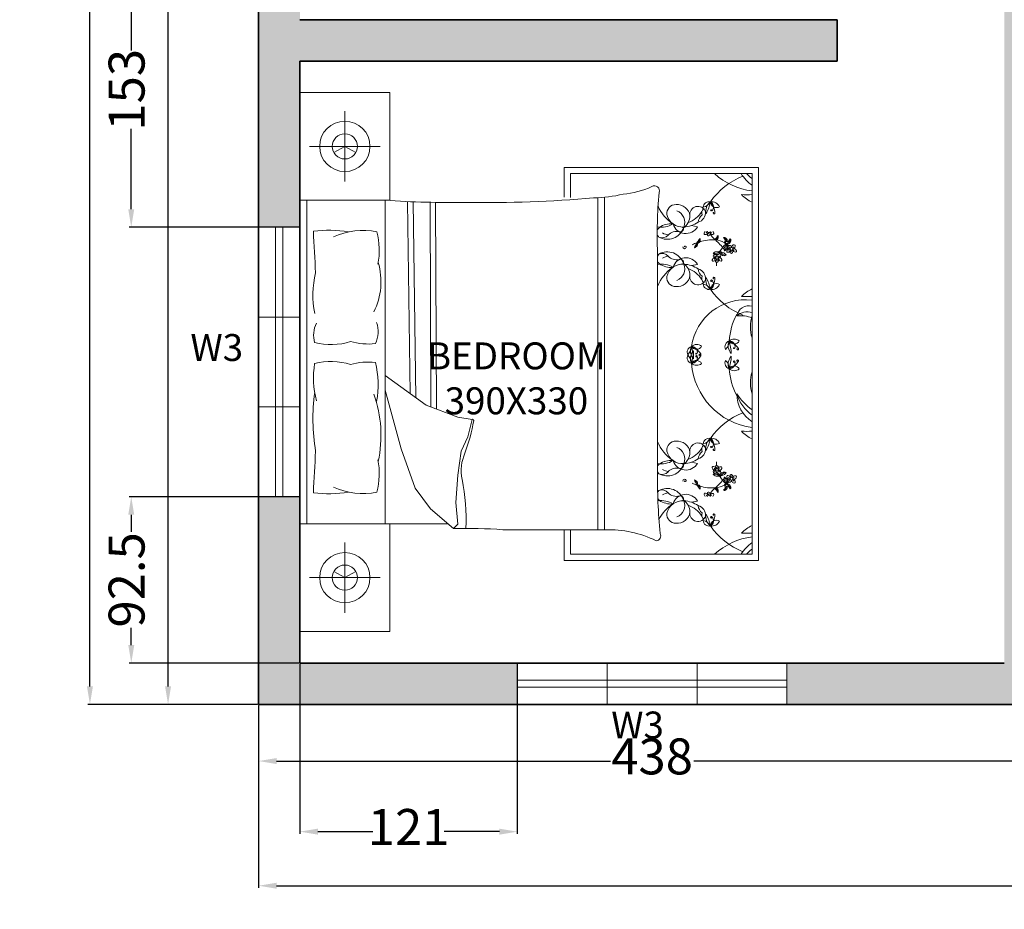
# Model space of a CAD drawing. Units: centimetres. Extents: x 2137 to 3697, y 183 to 2094.
# Tile 1 of 8: x 2137 to 2685, y 183 to 678. Entities that reach past the tile are written whole.
import ezdxf

# ---------------------------------------------------------------- set-up
doc = ezdxf.new("R2010")
doc.units = ezdxf.units.CM
for name, color, linetype, lineweight in [('A-ANNO-DIMS', 2, 'Continuous', 18), ('A-ANNO-TEXT', 7, 'Continuous', 18), ('A-AREA-IDEN', 7, 'Continuous', 25), ('A-FURN', 8, 'Continuous', 18), ('A-GLAZ', 4, 'Continuous', 18), ('A-WALL', 7, 'Continuous', 35), ('A-WALL-PATT', 52, 'Continuous', 13)]:
    doc.layers.add(name, color=color, linetype=linetype, lineweight=lineweight)
doc.styles.get("Standard").update_dxf_attribs({"font": 'arial.ttf'})
doc.dimstyles.new('ISO-25', dxfattribs={"dimtxt": 20, "dimasz": 10, "dimexe": 1.25, "dimexo": 0.625, "dimtad": 0, "dimtxsty": 'Standard', "dimcen": 2.5, "dimadec": 0, "dimazin": 0, "dimtfac": 1, "dimtmove": 0, "dimatfit": 3, "dimfxl": 1, "dimarcsym": 0})

# ---------------------------------------------------------------- blocks, each defined once
blk = doc.blocks.new('*D2')
at = {"layer": 'A-ANNO-DIMS', "color": 0, "lineweight": -2, "transparency": 16777216}
for p, q in [((2270.02, 295.95), (2270.02, 263.76)), ((2708.02, 295.95), (2708.02, 263.76)), ((2280.02, 265.01), (2465.88, 265.01)), ((2698.02, 265.01), (2512.16, 265.01))]:
    blk.add_line(p, q, dxfattribs=at)
at = {"layer": 'A-ANNO-DIMS', "color": 0, "transparency": 16777216}
for points in [[(2280.02, 266.68), (2280.02, 263.35), (2270.02, 265.01)], [(2698.02, 266.68), (2698.02, 263.35), (2708.02, 265.01)]]:
    blk.add_solid(points, dxfattribs=at)
at = {"layer": 'Defpoints', "color": 0, "transparency": 16777216}
for p in [(2270.02, 296.58), (2708.02, 296.58), (2708.02, 265.01)]:
    blk.add_point(p, dxfattribs=at)
at = {"layer": 'A-ANNO-DIMS', "color": 0, "transparency": 16777216, "insert": (2489.02, 265.01), "char_height": 20, "attachment_point": 5}
blk.add_mtext('438', dxfattribs=at)
blk = doc.blocks.new('*D5')
at = {"layer": 'A-ANNO-DIMS', "color": 0, "lineweight": -2, "transparency": 16777216}
for p, q in [((3590.02, 419.95), (3590.02, 194.39)), ((2270.02, 295.95), (2270.02, 194.39)), ((2280.02, 195.64), (2900.51, 195.64)), ((3580.02, 195.64), (2959.54, 195.64))]:
    blk.add_line(p, q, dxfattribs=at)
at = {"layer": 'A-ANNO-DIMS', "color": 0, "transparency": 16777216}
for points in [[(2280.02, 197.31), (2280.02, 193.97), (2270.02, 195.64)], [(3580.02, 197.31), (3580.02, 193.97), (3590.02, 195.64)]]:
    blk.add_solid(points, dxfattribs=at)
at = {"layer": 'Defpoints', "color": 0, "transparency": 16777216}
for p in [(3590.02, 420.58), (2270.02, 296.58), (3590.02, 195.64)]:
    blk.add_point(p, dxfattribs=at)
at = {"layer": 'A-ANNO-DIMS', "color": 0, "transparency": 16777216, "insert": (2930.02, 195.64), "char_height": 20, "attachment_point": 5}
blk.add_mtext('1320', dxfattribs=at)
blk = doc.blocks.new('*D7')
at = {"layer": 'A-ANNO-DIMS', "color": 0, "lineweight": -2, "transparency": 16777216}
for p, q in [((2269.4, 1526.58), (2218.41, 1526.58)), ((2219.66, 1516.58), (2219.66, 941.09)), ((2219.66, 306.58), (2219.66, 882.07)), ((2269.4, 296.58), (2218.41, 296.58))]:
    blk.add_line(p, q, dxfattribs=at)
at = {"layer": 'A-ANNO-DIMS', "color": 0, "transparency": 16777216}
for points in [[(2217.99, 1516.58), (2221.33, 1516.58), (2219.66, 1526.58)], [(2217.99, 306.58), (2221.33, 306.58), (2219.66, 296.58)]]:
    blk.add_solid(points, dxfattribs=at)
at = {"layer": 'Defpoints', "color": 0, "transparency": 16777216}
for p in [(2270.02, 1526.58), (2219.66, 296.58), (2270.02, 296.58)]:
    blk.add_point(p, dxfattribs=at)
at = {"layer": 'A-ANNO-DIMS', "color": 0, "transparency": 16777216, "insert": (2219.66, 911.58), "char_height": 20, "attachment_point": 5, "rotation": 90}
blk.add_mtext('1230', dxfattribs=at)
blk = doc.blocks.new('BED')
for p, q in [((2442.52, 2474.71), (2742.52, 2474.71)), ((2502.52, 2474.71), (2502.52, 2392.37)), ((2472.52, 2430.11), (2472.52, 2469.31)), ((2682.52, 2470.86), (2502.52, 2470.86)), ((2712.52, 2430.11), (2712.52, 2469.31)), ((2492.12, 2449.71), (2452.92, 2449.71)), ((2692.92, 2449.71), (2732.12, 2449.71)), ((2502.52, 2427.3), (2682.52, 2427.3)), ((2544.19, 2418.38), (2576.9, 2427.3)), ((2584.93, 2427.3), (2568.49, 2404.42)), ((2522.31, 2410.49), (2544.19, 2418.38)), ((2681.6, 2411.76), (2572.66, 2410.22)), ((2681.71, 2414.84), (2574.9, 2413.34)), ((2510.77, 2401.99), (2522.31, 2410.49)), ((2499.83, 2389.24), (2510.77, 2401.99)), ((2568.49, 2404.42), (2561.81, 2386.81)), ((2681.44, 2402.31), (2567.52, 2401.86)), ((2681.46, 2399.23), (2566.35, 2398.76)), ((2502.26, 2386.81), (2499.83, 2389.24)), ((2514.41, 2388.02), (2502.26, 2386.81)), ((2529.61, 2386.81), (2514.41, 2388.02)), ((2542.97, 2384.99), (2529.61, 2386.81)), ((2550.87, 2381.34), (2542.97, 2384.99)), ((2561.81, 2386.81), (2560.59, 2378.91)), ((2560.59, 2378.91), (2550.87, 2381.34)), ((2482.11, 2327.65), (2499.08, 2327.65)), ((2482.11, 2219.58), (2482.11, 2327.65)), ((2499.08, 2324.17), (2485.59, 2324.17)), ((2485.59, 2324.17), (2485.59, 2223.06)), ((2697.35, 2324.17), (2684.13, 2324.17)), ((2684.19, 2327.65), (2700.83, 2327.65)), ((2697.35, 2223.06), (2697.35, 2324.17)), ((2700.83, 2327.65), (2700.83, 2219.58)), ((2683.88, 2308.94), (2499.06, 2308.94)), ((2684.17, 2305.2), (2499.06, 2305.2)), ((2653.42, 2275.73), (2531.62, 2275.73)), ((2515.15, 2253.47), (2514.49, 2256.86)), ((2536.12, 2253.47), (2536.78, 2256.86)), ((2646.82, 2253.47), (2646.16, 2256.86)), ((2667.79, 2253.47), (2668.45, 2256.86)), ((2700.83, 2219.58), (2482.11, 2219.58)), ((2485.59, 2223.06), (2697.35, 2223.06))]:
    blk.add_line(p, q)
for points in [[(2502.52, 2424.71), (2442.52, 2424.71), (2442.52, 2474.71)], [(2682.52, 2474.71), (2682.52, 2424.71), (2742.52, 2424.71), (2742.52, 2474.71)], [(2472.52, 2449.71), (2476.02, 2455.77)], [(2712.52, 2449.71), (2709.02, 2455.77)], [(2472.52, 2449.71), (2476.02, 2443.65)], [(2712.52, 2449.71), (2709.02, 2443.65)]]:
    blk.add_lwpolyline(points)
for points in [[(2519.75, 2467.23, 0.074897), (2520.11, 2447.64, -0.472817)], [(2591.11, 2446.54, 0.14099), (2591.71, 2466.53, 0.235245)], [(2603.92, 2446.54, -0.14099), (2603.32, 2466.53, -0.235245)], [(2665.29, 2467.23, -0.074897), (2664.92, 2447.64, 0.472817)], [(2499.2, 2361.77, 0.001242), (2499.06, 2304.85, -0.127202), (2493.05, 2276.48)], [(2683.8, 2311.3, 0.056112), (2685.97, 2294.79, 0.095341), (2690.19, 2278.9)]]:
    blk.add_lwpolyline(points, format="xyb")
for centre, radius in [((2472.52, 2449.71), 14), ((2712.52, 2449.71), 14), ((2472.52, 2449.71), 7), ((2712.52, 2449.71), 7), ((2532.49, 2242.6), 0.764), ((2650.46, 2242.6), 0.764), ((2527.49, 2234.55), 0.764), ((2655.45, 2234.55), 0.764)]:
    blk.add_circle(centre, radius)
for centre, radius, start, end in [((2685.11, 5322.24), 2859.79, 266.68521, 267.14978), ((2560.85, 2358.67), 108.8, 82.2196, 99.497), ((2583.83, 2413.66), 53.46, 81.5249, 103.96), ((2607.44, 2452.27), 14.84, 63.3437, 106.1026), ((2629.68, 2414.74), 52.74, 76.3427, 101.1841), ((2499.93, 5322.24), 2859.79, 272.85022, 273.31479), ((2557.97, 2439.77), 38.67, 155.1316, 191.7583), ((2627.07, 2439.77), 38.67, 348.2417, 24.8684), ((2555.75, 2436.51), 36.76, 354.0129, 15.8293), ((2639.29, 2436.51), 36.76, 164.1707, 185.9871), ((2551.61, 2499.32), 69.73, 258.0397, 289.2615), ((2637.23, 2467.78), 38.19, 243.8761, 286.1746), ((2530.45, 2470.74), 40.2, 255.1039, 281.0369), ((2579.84, 2484.1), 52.9, 259.8617, 283.6238), ((2609.45, 2447.1), 15.9, 245.0183, 288.5407), ((2654.58, 2470.74), 40.2, 258.9631, 284.8961), ((3220.32, 2390.64), 539.05, 176.1, 180.9282), ((2224.76, 2381.78), 275.17, 355.8294, 1.553), ((2504.97, 2495.47), 113.22, 267.4519, 281.3392), ((2532.03, 2360.52), 24.42, 66.2616, 101.3392), ((2581.42, 2492.28), 116.34, 250.1194, 259.3383), ((2559.91, 2378.67), 0.724, 268.8623, 19.7536), ((3384.42, 2371.04), 703.17, 179.11454, 184.87351), ((2495.81, 2276.67), 2.77, 183.98, 297.3412), ((2528.04, 1963.45), 312.3, 89.3433, 95.6887), ((2494.64, 2254.6), 22.71, 33.6671, 63.2997), ((2525.07, 2268.11), 11.57, 145.785, 184.7304), ((2502.97, 2273.51), 12.43, 328.8218, 9.1554), ((2518.36, 2272.41), 3.61, 120.0293, 142.325), ((2512.59, 2270.28), 9.56, 289.2822, 29.1751), ((2516.83, 2273.13), 4.49, 311.5653, 23.8354), ((2518.36, 2272.41), 3.61, 44.4517, 63.558), ((2538.68, 2270.28), 9.56, 150.8249, 250.7178), ((2534.44, 2273.13), 4.49, 156.1646, 228.4347), ((2532.91, 2272.41), 3.61, 113.229, 135.5483), ((2532.91, 2272.41), 3.61, 37.675, 66.7144), ((2526.21, 2268.11), 11.57, 355.2696, 34.215), ((2548.31, 2273.51), 12.43, 169.7133, 211.1782), ((2556.64, 2254.6), 22.71, 111.4941, 146.3329), ((2626.3, 2254.6), 22.71, 33.6671, 68.5059), ((2656.73, 2268.11), 11.57, 145.785, 184.7304), ((2634.63, 2273.51), 12.43, 328.8218, 10.2867), ((2650.03, 2272.41), 3.61, 113.2856, 142.325), ((2644.26, 2270.28), 9.56, 289.2822, 29.1751), ((2650.03, 2272.41), 3.61, 44.4517, 66.7144), ((2648.5, 2273.13), 4.49, 311.5653, 23.8354), ((2662.61, 1983.95), 291.92, 85.2402, 91.8035), ((2670.35, 2270.28), 9.56, 150.8249, 250.7178), ((2666.11, 2273.13), 4.49, 156.1646, 228.4347), ((2664.58, 2272.41), 3.61, 106.6343, 135.5483), ((2664.58, 2272.41), 3.61, 37.675, 72.5814), ((2657.87, 2268.11), 11.57, 355.2696, 34.215), ((2679.98, 2273.51), 12.43, 169.249, 211.1782), ((2688.3, 2254.6), 22.71, 113.6453, 146.3329), ((2687.92, 2277.37), 2.73, 246.5219, 33.8264), ((2507.86, 2265.5), 5.07, 84.4856, 181.0538), ((2506.31, 2261.76), 9.02, 355.2933, 76.921), ((2523.89, 2265.16), 6.15, 131.5653, 195.1471), ((2511.15, 2268.55), 8.62, 7.436, 29.9149), ((2527.38, 2265.16), 6.15, 344.8529, 48.4347), ((2540.13, 2268.55), 8.62, 150.0851, 172.564), ((2544.97, 2261.76), 9.02, 103.079, 184.7067), ((2543.41, 2265.5), 5.07, 358.9462, 95.5144), ((2639.53, 2265.5), 5.07, 84.4856, 181.0538), ((2637.98, 2261.76), 9.02, 355.2933, 76.921), ((2655.56, 2265.16), 6.15, 131.5653, 195.1471), ((2642.81, 2268.55), 8.62, 7.436, 29.9149), ((2659.05, 2265.16), 6.15, 344.8529, 48.4347), ((2671.79, 2268.55), 8.62, 150.0851, 172.564), ((2676.63, 2261.76), 9.02, 103.079, 184.7067), ((2675.08, 2265.5), 5.07, 358.9462, 95.5144), ((2509.94, 2264.78), 7.17, 174.9449, 262.8857), ((2512.76, 2267.5), 6.96, 201.5819, 291.4221), ((2511.44, 2259.94), 7.46, 299.9085, 73.1337), ((2516.16, 2263.07), 1.86, 257.3041, 15.1471), ((2539.84, 2259.94), 7.46, 106.8663, 240.0915), ((2535.12, 2263.07), 1.86, 164.8529, 282.6959), ((2538.52, 2267.5), 6.96, 248.5779, 338.4181), ((2541.33, 2264.78), 7.17, 277.1143, 5.0551), ((2641.61, 2264.78), 7.17, 174.9449, 262.8857), ((2644.43, 2267.5), 6.96, 201.5819, 291.4221), ((2643.1, 2259.94), 7.46, 299.9085, 73.1337), ((2647.82, 2263.07), 1.86, 257.3041, 15.1471), ((2671.51, 2259.94), 7.46, 106.8663, 240.0915), ((2666.78, 2263.07), 1.86, 164.8529, 282.6959), ((2670.18, 2267.5), 6.96, 248.5779, 338.4181), ((2673, 2264.78), 7.17, 277.1143, 5.0551), ((2508.29, 2253.23), 4.5, 80.264, 250.8688), ((2499.37, 2263.14), 14.16, 301.2614, 341.7045), ((2508.7, 2266.37), 8.71, 272.3591, 324.0401), ((2499.23, 2262), 16.1, 326.2883, 356.5076), ((2525.07, 2268.11), 11.57, 212.7011, 216.3445), ((2526.5, 2260.25), 0.578, 102.7051, 280.4384), ((2526.43, 2260.6), 0.94, 280.4384, 100.4136), ((2526.21, 2268.11), 11.57, 323.6555, 327.2989), ((2542.58, 2266.37), 8.71, 215.9599, 267.6409), ((2552.04, 2262), 16.1, 183.4924, 213.7117), ((2551.91, 2263.14), 14.16, 198.2955, 238.7386), ((2542.98, 2253.23), 4.5, 289.1312, 99.736), ((2594.92, 2255.93), 3.25, 63.0274, 163.8037), ((2591.63, 2263.52), 6.69, 271.4585, 315.3727), ((2598.02, 2255.93), 3.25, 16.1963, 116.9726), ((2601.31, 2263.52), 6.69, 224.6273, 268.5415), ((2639.96, 2253.23), 4.5, 80.264, 250.8688), ((2631.03, 2263.14), 14.16, 301.2614, 341.7045), ((2640.36, 2266.37), 8.71, 272.3591, 324.0401), ((2630.9, 2262), 16.1, 326.2883, 356.5076), ((2656.73, 2268.11), 11.57, 212.7011, 216.3445), ((2656.51, 2260.6), 0.94, 79.5864, 259.5616), ((2656.44, 2260.25), 0.578, 259.5616, 77.2949), ((2657.87, 2268.11), 11.57, 323.6555, 327.2989), ((2674.25, 2266.37), 8.71, 215.9599, 267.6409), ((2683.71, 2262), 16.1, 183.4924, 213.7117), ((2683.58, 2263.14), 14.16, 198.2955, 238.7386), ((2674.65, 2253.23), 4.5, 289.1312, 99.736), ((2507.21, 2254.58), 5.62, 265.969, 344.3045), ((2513.27, 2247.11), 5.99, 96.1662, 141.5825), ((2523.19, 2251.31), 1.58, 101.3256, 154.4621), ((2520.92, 2256.65), 4.74, 280.2588, 300.656), ((2522.01, 2260.45), 8.46, 268.3264, 277.1302), ((2547.29, 2245.15), 24.85, 163.5842, 183.8277), ((2519.89, 2256.64), 4.82, 308.2101, 316.3071), ((2522.85, 2253.47), 1.44, 278.3432, 4.2869), ((2522.06, 2254.74), 2.51, 300.656, 332.6341), ((2523.94, 2253.08), 0.611, 55.7657, 157.4417), ((2547.29, 2245.15), 24.85, 153.0032, 159.8941), ((2524.9, 2253.65), 0.611, 84.3784, 186.0543), ((2524.32, 2256.1), 2.51, 269.1859, 301.164), ((2525.06, 2254.8), 1.44, 237.5332, 323.4768), ((2523.67, 2258.9), 4.82, 285.5129, 293.6099), ((2526.81, 2253.48), 1.58, 87.3579, 140.4944), ((2523.17, 2258), 4.74, 301.164, 321.5612), ((2519.31, 2258.83), 8.46, 324.6898, 333.4936), ((2538.01, 2247.11), 5.99, 38.4175, 83.8338), ((2544.06, 2254.58), 5.62, 195.6955, 274.031), ((2594.85, 2217.78), 39.18, 94.4623, 172.255), ((2595.02, 2253.92), 4.34, 137.7873, 219.1145), ((2590.09, 2254.05), 3.27, 298.5391, 58.3627), ((2594.35, 2251.19), 6.19, 45.5411, 114.3101), ((2600, 2282.98), 27.41, 252.593, 267.2582), ((2595, 2256.71), 3.2, 177.7585, 283.852), ((2601.17, 2260.05), 9.91, 198.9159, 238.011), ((2598.59, 2251.19), 6.19, 65.6899, 134.4589), ((2592.94, 2282.98), 27.41, 272.7418, 287.407), ((2595.67, 2254.01), 0.424, 283.852, 219.9245), ((2596.18, 2252.06), 0.487, 238.011, 71.5592), ((2596.26, 2252.29), 0.236, 71.5592, 188.0167), ((2596.76, 2252.06), 0.487, 108.4408, 301.989), ((2596.68, 2252.29), 0.236, 351.9833, 108.4408), ((2597.23, 2254.17), 0.255, 320.1909, 256.0209), ((2591.77, 2260.05), 9.91, 301.989, 341.0841), ((2597.94, 2256.71), 3.2, 256.148, 2.2415), ((2602.86, 2254.05), 3.27, 121.6373, 241.4609), ((2597.92, 2253.92), 4.34, 320.8855, 42.2127), ((2596.83, 2226.82), 30.32, 352.8636, 81.8197), ((2638.88, 2254.58), 5.62, 265.969, 344.3045), ((2644.93, 2247.11), 5.99, 96.1662, 141.5825), ((2656.13, 2253.48), 1.58, 39.5056, 92.6421), ((2659.77, 2258), 4.74, 218.4388, 238.836), ((2663.63, 2258.83), 8.46, 206.5064, 215.3102), ((2657.88, 2254.8), 1.44, 216.5232, 302.4668), ((2658.62, 2256.1), 2.51, 238.836, 270.8141), ((2659.27, 2258.9), 4.82, 246.3901, 254.4871), ((2635.65, 2245.15), 24.85, 20.1059, 26.9968), ((2658.05, 2253.65), 0.611, 353.9457, 95.6216), ((2659, 2253.08), 0.611, 22.5583, 124.2343), ((2660.09, 2253.47), 1.44, 175.7131, 261.6568), ((2660.89, 2254.74), 2.51, 207.3659, 239.344), ((2635.65, 2245.15), 24.85, 356.1723, 16.4158), ((2663.05, 2256.64), 4.82, 223.6929, 231.7899), ((2662.02, 2256.65), 4.74, 239.344, 259.7412), ((2660.93, 2260.45), 8.46, 262.8698, 271.6736), ((2659.76, 2251.31), 1.58, 25.5379, 78.6744), ((2675.73, 2254.58), 5.62, 195.6955, 274.031), ((2669.67, 2247.11), 5.99, 38.4175, 83.8338), ((2504.48, 2247), 3.25, 92.9516, 193.728), ((2497.84, 2251.95), 6.69, 301.3827, 345.2969), ((2506.35, 2242.61), 6.19, 75.4653, 144.2343), ((2495.38, 2272.99), 27.41, 282.5173, 297.1824), ((2507.37, 2248.35), 2.76, 63.9755, 143.2681), ((2518.73, 2248.32), 1.27, 101.5637, 142.6358), ((2517.68, 2247.14), 0.764, 273.2768, 86.7232), ((2518.57, 2247.86), 0.73, 91.1081, 181.8675), ((2519.34, 2246.4), 1.58, 80.3487, 133.6538), ((2519.06, 2247.7), 1.25, 229.7889, 317.6792), ((2517.71, 2249.32), 1.84, 288.7263, 352.5032), ((2517.65, 2245.06), 1.78, 355.053, 68.3618), ((2519.04, 2244.75), 2.5, 83.0852, 105.7171), ((2518.96, 2249.23), 0.59, 345.2356, 144.9248), ((2519.5, 2247.3), 0.658, 317.6792, 80.3487), ((2543.91, 2248.35), 2.76, 36.7319, 116.0245), ((2544.93, 2242.61), 6.19, 35.7657, 104.5347), ((2555.89, 2272.99), 27.41, 242.8176, 257.4827), ((2546.8, 2247), 3.25, 346.272, 87.0484), ((2553.44, 2251.95), 6.69, 194.7031, 238.6173), ((2636.14, 2247), 3.25, 92.9516, 193.728), ((2629.51, 2251.95), 6.69, 301.3827, 345.2969), ((2638.02, 2242.61), 6.19, 75.4653, 144.2343), ((2627.05, 2272.99), 27.41, 282.5173, 297.1824), ((2639.03, 2248.35), 2.76, 63.9755, 143.2681), ((2663.45, 2247.3), 0.658, 99.6513, 222.3208), ((2663.88, 2247.7), 1.25, 222.3208, 310.2111), ((2663.6, 2246.4), 1.58, 46.3462, 99.6513), ((2663.98, 2249.23), 0.59, 35.0752, 194.7644), ((2665.23, 2249.32), 1.84, 187.4968, 251.2737), ((2665.29, 2245.06), 1.78, 111.6382, 184.947), ((2663.9, 2244.75), 2.5, 74.2829, 96.9148), ((2664.38, 2247.86), 0.73, 358.1325, 88.8919), ((2664.21, 2248.32), 1.27, 37.3642, 78.4363), ((2665.27, 2247.14), 0.764, 93.2768, 266.7232), ((2675.58, 2248.35), 2.76, 36.7319, 116.0245), ((2676.59, 2242.61), 6.19, 35.7657, 104.5347), ((2687.56, 2272.99), 27.41, 242.8176, 257.4827), ((2685.1, 2251.95), 6.69, 194.7031, 238.6173), ((2678.46, 2247), 3.25, 346.272, 87.0484), ((2456.43, 2217.78), 39.18, 7.745, 41.8856), ((2523.45, 2213.9), 39.18, 124.3865, 158.5908), ((2505.57, 2245.31), 4.34, 167.7115, 249.0387), ((2501.23, 2242.96), 3.27, 328.4633, 88.2869), ((2507.84, 2253.69), 9.91, 228.8402, 267.9352), ((2504.16, 2247.72), 3.2, 207.6827, 313.7762), ((2506.09, 2245.71), 0.424, 313.7762, 249.7183), ((2507.46, 2244.52), 0.236, 101.4834, 217.9409), ((2507.5, 2244.28), 0.487, 267.9352, 101.4834), ((2518.72, 2245.73), 1.26, 217.7621, 259.0403), ((2520.08, 2247.41), 2.32, 203.4276, 227.6104), ((2518.83, 2244.95), 0.586, 232.4737, 355.053), ((2501.72, 2224.01), 28.48, 43.1541, 52.0459), ((2521.4, 2241.21), 1.58, 101.3256, 154.4621), ((2519.13, 2246.56), 4.74, 280.2588, 300.656), ((2520.22, 2250.35), 8.46, 268.3264, 277.1302), ((2518.11, 2246.55), 4.82, 308.2101, 316.3071), ((2521.07, 2243.38), 1.44, 278.3432, 4.2869), ((2520.27, 2244.64), 2.51, 300.656, 332.6341), ((2522.16, 2242.98), 0.611, 55.7657, 157.4417), ((2534.91, 2244.52), 12.46, 184.756, 209.2041), ((2552.85, 2271.04), 40.99, 222.2412, 232.1744), ((2528.5, 2242.96), 2.12, 272.8499, 356.1226), ((2526.64, 2243.74), 3.48, 304.5369, 16.3699), ((2527, 2242.14), 2.05, 321.7607, 7.9252), ((2531.47, 2242.76), 2.46, 127.3105, 187.9252), ((2528.09, 2243.04), 2.53, 355.0106, 41.658), ((2530.88, 2241.17), 0.757, 148.0499, 225.6268), ((2536.2, 2227.98), 14.94, 113.0501, 113.8477), ((2532.28, 2240.29), 2.41, 104.7558, 148.0499), ((2530.93, 2242.02), 1.51, 247.4086, 351.4386), ((2531.64, 2243.66), 1.04, 126.1046, 271.4281), ((2531.53, 2243.95), 0.749, 353.7526, 131.7054), ((2531.35, 2241.96), 0.506, 262.906, 7.132), ((2530.82, 2243.06), 1.05, 0.0645, 61.1507), ((2531.07, 2243.95), 1.2, 311.8413, 355.7877), ((2533.54, 2243.78), 1.27, 101.5637, 176.365), ((2533.53, 2241.19), 1.26, 151.2196, 259.0403), ((2533.38, 2243.32), 0.73, 91.1081, 181.8675), ((2534.89, 2242.87), 2.32, 203.4276, 227.6104), ((2534.15, 2241.86), 1.58, 80.3487, 133.6538), ((2533.87, 2243.16), 1.25, 229.7889, 317.6792), ((2532.52, 2244.78), 1.84, 288.7263, 352.5032), ((2532.46, 2240.51), 1.78, 355.053, 68.3618), ((2533.85, 2240.21), 2.5, 83.0852, 105.7171), ((2533.77, 2244.69), 0.59, 345.2356, 144.9248), ((2534.31, 2242.76), 0.658, 317.6792, 80.3487), ((2536.2, 2227.98), 14.94, 87.1071, 94.7585), ((2543.77, 2244.28), 0.487, 78.5166, 272.0648), ((2543.43, 2253.69), 9.91, 272.0648, 311.1598), ((2543.82, 2244.52), 0.236, 322.0591, 78.5166), ((2547.11, 2247.72), 3.2, 226.2238, 332.3173), ((2545.24, 2245.88), 0.255, 290.2667, 226.2271), ((2550.05, 2242.96), 3.27, 91.7131, 211.5367), ((2545.71, 2245.31), 4.34, 290.9613, 12.2885), ((2527.83, 2213.9), 39.18, 21.4092, 55.6135), ((2655.12, 2213.9), 39.18, 124.3865, 158.5908), ((2637.23, 2245.31), 4.34, 167.7115, 249.0387), ((2635.83, 2247.72), 3.2, 207.6827, 313.7762), ((2639.51, 2253.69), 9.91, 228.8402, 267.9352), ((2632.89, 2242.96), 3.27, 328.4633, 88.2869), ((2637.75, 2245.71), 0.424, 313.7762, 249.7183), ((2639.12, 2244.52), 0.236, 101.4834, 217.9409), ((2639.17, 2244.28), 0.487, 267.9352, 101.4834), ((2646.75, 2227.98), 14.94, 85.2415, 92.8929), ((2648.64, 2242.76), 0.658, 99.6513, 222.3208), ((2649.07, 2243.16), 1.25, 222.3208, 310.2111), ((2648.79, 2241.86), 1.58, 46.3462, 99.6513), ((2649.17, 2244.69), 0.59, 35.0752, 194.7644), ((2650.42, 2244.78), 1.84, 187.4968, 251.2737), ((2650.48, 2240.51), 1.78, 111.6382, 184.947), ((2649.09, 2240.21), 2.5, 74.2829, 96.9148), ((2649.56, 2243.32), 0.73, 358.1325, 88.8919), ((2648.05, 2242.87), 2.32, 312.3896, 336.5724), ((2649.4, 2243.78), 1.27, 3.635, 78.4363), ((2649.41, 2241.19), 1.26, 280.9597, 28.7804), ((2652.01, 2242.02), 1.51, 188.5614, 292.5914), ((2651.41, 2243.95), 0.749, 48.2946, 186.2474), ((2651.87, 2243.95), 1.2, 184.2123, 228.1587), ((2652.12, 2243.06), 1.05, 118.8493, 179.9355), ((2651.59, 2241.96), 0.506, 172.868, 277.094), ((2651.3, 2243.66), 1.04, 268.5719, 53.8954), ((2650.66, 2240.29), 2.41, 31.9501, 75.2442), ((2654.85, 2243.04), 2.53, 138.342, 184.9894), ((2654.44, 2242.96), 2.12, 183.8774, 267.1501), ((2652.06, 2241.17), 0.757, 314.3732, 31.9501), ((2646.75, 2227.98), 14.94, 66.1523, 66.9499), ((2656.3, 2243.74), 3.48, 163.6301, 235.4631), ((2651.47, 2242.76), 2.46, 352.0748, 52.6895), ((2655.94, 2242.14), 2.05, 172.0748, 218.2393), ((2630.09, 2271.04), 40.99, 307.8256, 317.7588), ((2648.03, 2244.52), 12.46, 330.7959, 355.244), ((2681.22, 2224.01), 28.48, 127.9541, 136.8459), ((2660.78, 2242.98), 0.611, 22.5583, 124.2343), ((2661.88, 2243.38), 1.44, 175.7131, 261.6568), ((2662.67, 2244.64), 2.51, 207.3659, 239.344), ((2664.83, 2246.55), 4.82, 223.6929, 231.7899), ((2663.81, 2246.56), 4.74, 239.344, 259.7412), ((2662.72, 2250.35), 8.46, 262.8698, 271.6736), ((2661.54, 2241.21), 1.58, 25.5379, 78.6744), ((2664.11, 2244.95), 0.586, 184.947, 307.5263), ((2662.86, 2247.41), 2.32, 312.3896, 336.5724), ((2664.23, 2245.73), 1.26, 280.9597, 322.2379), ((2675.44, 2244.28), 0.487, 78.5166, 272.0648), ((2675.1, 2253.69), 9.91, 272.0648, 311.1598), ((2675.49, 2244.52), 0.236, 322.0591, 78.5166), ((2678.78, 2247.72), 3.2, 226.2238, 332.3173), ((2676.9, 2245.88), 0.255, 290.2667, 226.2271), ((2681.72, 2242.96), 3.27, 91.7131, 211.5367), ((2677.37, 2245.31), 4.34, 290.9613, 12.2885), ((2659.49, 2213.9), 39.18, 21.4092, 55.6135), ((2726.52, 2217.78), 39.18, 138.1144, 172.255), ((2521.93, 2238.45), 0.853, 146.8636, 236.9021), ((2533.96, 2257.24), 22.32, 235.1882, 238.8844), ((2523.39, 2239.69), 2.31, 199.4799, 267.6828), ((2523.14, 2238.82), 1.99, 212.8155, 277.3992), ((2521.98, 2237.49), 2.31, 266.9701, 338.2913), ((2509.81, 2253.97), 22.32, 302.6784, 306.3746), ((2522.88, 2238.89), 0.883, 238.8844, 314.2646), ((2522.69, 2236.91), 1.99, 280.3057, 17.1958), ((2522.52, 2236.71), 0.883, 306.3746, 21.7548), ((2523.96, 2237.28), 0.666, 19.3605, 201.7548), ((2523.96, 2237.78), 0.666, 311.8703, 134.2646), ((2536.49, 2231.71), 13.31, 153.7819, 158.2913), ((2525.9, 2240.8), 3.48, 247.2305, 319.0635), ((2524.75, 2239.63), 2.05, 264.4544, 310.6188), ((2534.91, 2244.52), 12.46, 214.0033, 222.4917), ((2526.25, 2238.81), 2.12, 218.3208, 298.8162), ((2536.2, 2227.98), 14.94, 120.544, 139.818), ((2526.65, 2235.61), 1.04, 126.1046, 271.4281), ((2526.53, 2235.89), 0.749, 353.7526, 131.7054), ((2527.69, 2236.2), 2.46, 70.0041, 130.6188), ((2525.83, 2235), 1.05, 0.0645, 61.1507), ((2526.08, 2235.9), 1.2, 311.8413, 355.7877), ((2526.09, 2239.2), 2.53, 297.7043, 344.3516), ((2528.55, 2235.73), 1.27, 101.5637, 176.365), ((2528.38, 2235.27), 0.73, 91.1081, 181.8675), ((2527.52, 2236.73), 1.84, 288.7263, 352.5032), ((2528.77, 2236.64), 0.59, 345.2356, 144.9248), ((2527.43, 2239.19), 2.05, 8.7227, 54.8872), ((2527.54, 2237.55), 3.48, 0.278, 72.111), ((2529.1, 2238.83), 2.12, 20.5253, 88.5375), ((2531.89, 2239.88), 2.46, 188.7227, 249.3375), ((2528.73, 2238.64), 2.53, 334.9899, 21.6373), ((2533.64, 2240.41), 0.586, 232.4737, 355.053), ((2591.85, 2196.79), 39.18, 94.4623, 117.4146), ((2592.02, 2232.93), 4.34, 137.7873, 219.1145), ((2587.09, 2233.07), 3.27, 298.5391, 58.3627), ((2591.92, 2234.94), 3.25, 63.0274, 163.8037), ((2588.63, 2242.54), 6.69, 271.4585, 315.3727), ((2591.35, 2230.21), 6.19, 45.5411, 114.3101), ((2598.17, 2239.06), 9.91, 198.9159, 238.011), ((2597, 2262), 27.41, 252.593, 267.2582), ((2592, 2235.73), 3.2, 177.7585, 283.852), ((2601.59, 2230.21), 6.19, 65.6899, 134.4589), ((2595.94, 2262), 27.41, 272.7418, 287.407), ((2601.02, 2234.94), 3.25, 16.1963, 116.9726), ((2604.31, 2242.54), 6.69, 224.6273, 268.5415), ((2594.77, 2239.06), 9.91, 301.989, 341.0841), ((2600.94, 2235.73), 3.2, 256.148, 2.2415), ((2605.86, 2233.07), 3.27, 121.6373, 241.4609), ((2600.92, 2232.93), 4.34, 320.8855, 42.2127), ((2601.09, 2196.79), 39.18, 62.5854, 85.5377), ((2649.3, 2240.41), 0.586, 184.947, 307.5263), ((2654.21, 2238.64), 2.53, 158.3627, 205.0101), ((2653.84, 2238.83), 2.12, 91.4625, 159.4747), ((2655.4, 2237.55), 3.48, 107.889, 179.722), ((2651.05, 2239.88), 2.46, 290.6625, 351.2773), ((2655.51, 2239.19), 2.05, 125.1128, 171.2773), ((2654.17, 2236.64), 0.59, 35.0752, 194.7644), ((2655.42, 2236.73), 1.84, 187.4968, 251.2737), ((2646.75, 2227.98), 14.94, 40.182, 59.456), ((2655.26, 2236.2), 2.46, 49.3812, 109.9959), ((2657.04, 2240.8), 3.48, 220.9365, 292.7695), ((2656.85, 2239.2), 2.53, 195.6484, 242.2957), ((2654.56, 2235.27), 0.73, 358.1325, 88.8919), ((2654.4, 2235.73), 1.27, 3.635, 78.4363), ((2656.41, 2235.89), 0.749, 48.2946, 186.2474), ((2656.69, 2238.81), 2.12, 241.1838, 321.6792), ((2656.87, 2235.9), 1.2, 184.2123, 228.1587), ((2657.12, 2235), 1.05, 118.8493, 179.9355), ((2656.3, 2235.61), 1.04, 268.5719, 53.8954), ((2658.19, 2239.63), 2.05, 229.3812, 275.5456), ((2648.03, 2244.52), 12.46, 317.5083, 325.9967), ((2660.25, 2236.91), 1.99, 162.8042, 259.6943), ((2658.98, 2237.78), 0.666, 45.7354, 228.1297), ((2658.98, 2237.28), 0.666, 338.2452, 160.6395), ((2646.45, 2231.71), 13.31, 21.7087, 26.2181), ((2660.96, 2237.49), 2.31, 201.7087, 273.0299), ((2660.06, 2238.89), 0.883, 225.7354, 301.1156), ((2660.42, 2236.71), 0.883, 158.2452, 233.6254), ((2659.81, 2238.82), 1.99, 262.6008, 327.1845), ((2659.55, 2239.69), 2.31, 272.3172, 340.5201), ((2673.14, 2253.97), 22.32, 233.6254, 237.3216), ((2648.98, 2257.24), 22.32, 301.1156, 304.8118), ((2661.01, 2238.45), 0.853, 303.0979, 33.1364), ((2522.56, 2235.66), 0.853, 214.3538, 304.3923), ((2525.88, 2233.11), 0.757, 148.0499, 225.6268), ((2527.28, 2232.24), 2.41, 104.7558, 148.0499), ((2525.93, 2233.96), 1.51, 247.4086, 351.4386), ((2526.36, 2233.9), 0.506, 262.906, 7.132), ((2528.53, 2233.13), 1.26, 151.2196, 259.0403), ((2529.89, 2234.81), 2.32, 203.4276, 227.6104), ((2529.15, 2233.8), 1.58, 80.3487, 133.6538), ((2528.87, 2235.11), 1.25, 229.7889, 317.6792), ((2527.46, 2232.46), 1.78, 355.053, 68.3618), ((2528.85, 2232.16), 2.5, 83.0852, 105.7171), ((2528.65, 2232.36), 0.586, 232.4737, 355.053), ((2529.31, 2234.71), 0.658, 317.6792, 80.3487), ((2575.2, 2212.53), 19.09, 91.272, 146.5383), ((2582.06, 2208.97), 23.79, 107.8504, 143.6964), ((2594.57, 2202.28), 35.39, 124.0123, 144.053), ((2592.67, 2233.03), 0.424, 283.852, 219.9245), ((2593.18, 2231.07), 0.487, 238.011, 71.5592), ((2593.26, 2231.31), 0.236, 71.5592, 188.0167), ((2599.76, 2231.07), 0.487, 108.4408, 301.989), ((2599.68, 2231.31), 0.236, 351.9833, 108.4408), ((2600.23, 2233.19), 0.255, 320.1909, 256.0209), ((2600.75, 2229.59), 17.54, 338.117, 6.6195), ((2616.84, 2224.71), 7.03, 346.3898, 79.0739), ((2611.55, 2225.68), 8.89, 342.8609, 41.9049), ((2653.63, 2234.71), 0.658, 99.6513, 222.3208), ((2654.07, 2235.11), 1.25, 222.3208, 310.2111), ((2653.79, 2233.8), 1.58, 46.3462, 99.6513), ((2655.48, 2232.46), 1.78, 111.6382, 184.947), ((2654.29, 2232.36), 0.586, 184.947, 307.5263), ((2654.09, 2232.16), 2.5, 74.2829, 96.9148), ((2653.05, 2234.81), 2.32, 312.3896, 336.5724), ((2654.41, 2233.13), 1.26, 280.9597, 28.7804), ((2657.01, 2233.96), 1.51, 188.5614, 292.5914), ((2656.58, 2233.9), 0.506, 172.868, 277.094), ((2655.66, 2232.24), 2.41, 31.9501, 75.2442), ((2657.06, 2233.11), 0.757, 314.3732, 31.9501), ((2660.38, 2235.66), 0.853, 235.6077, 325.6462), ((2476.08, 2212.53), 19.09, 33.4617, 60.1116), ((2469.21, 2208.97), 23.79, 36.3036, 46.4814), ((2486.77, 2216.95), 15.93, 22.5547, 48.9546), ((2443.14, 2225.51), 54.2, 357.4081, 3.6519), ((2564.51, 2216.95), 15.93, 131.0454, 157.4453), ((2608.14, 2225.51), 54.2, 176.3481, 182.5919), ((2574.8, 2225.51), 54.2, 357.4081, 3.6519), ((2618.44, 2216.95), 15.93, 22.5547, 48.9546), ((2696.17, 2216.95), 15.93, 131.0454, 157.4453), ((2739.8, 2225.51), 54.2, 176.3481, 182.5919), ((2706.86, 2212.53), 19.09, 119.8884, 146.5383), ((2713.73, 2208.97), 23.79, 133.5186, 143.6964), ((2580.89, 2202.46), 21.54, 73.5431, 107.0202), ((2589.43, 2191.36), 31.85, 94.3787, 95.6357), ((2606.21, 2169.53), 56.92, 109.7217, 109.9028), ((2612.05, 2202.46), 21.54, 72.9798, 106.4569), ((2603.51, 2191.36), 31.85, 84.3643, 85.6213), ((2586.74, 2169.53), 56.92, 70.0972, 70.2783)]:
    blk.add_arc(centre, radius, start, end)
blk = doc.blocks.new('WIN-W3-150CM')
for p, q in [((0, 23), (0, 0)), ((50, 23), (50, 0)), ((100, 23), (100, 0)), ((150, 23), (150, 0)), ((0, 13.5), (150, 13.5)), ((0, 9.5), (150, 9.5))]:
    blk.add_line(p, q)
blk = doc.blocks.new('*D24')
at = {"layer": 'A-ANNO-DIMS', "color": 0, "lineweight": -2, "transparency": 16777216}
for p, q in [((2293.02, 731.82), (2293.02, 720.04)), ((2367.34, 731.82), (2367.34, 720.04)), ((2293.02, 721.29), (2283.02, 721.29)), ((2357.34, 721.29), (2303.02, 721.29))]:
    blk.add_line(p, q, dxfattribs=at)
at = {"layer": 'A-ANNO-DIMS', "color": 0, "transparency": 16777216}
for points in [[(2303.02, 722.96), (2303.02, 719.63), (2293.02, 721.29)], [(2357.34, 722.96), (2357.34, 719.63), (2367.34, 721.29)]]:
    blk.add_solid(points, dxfattribs=at)
at = {"layer": 'Defpoints', "color": 0, "transparency": 16777216}
for p in [(2293.02, 732.44), (2367.34, 732.44), (2293.02, 721.29)]:
    blk.add_point(p, dxfattribs=at)
at = {"layer": 'A-ANNO-DIMS', "color": 0, "transparency": 16777216, "insert": (2206.16, 721.29), "char_height": 20, "attachment_point": 5}
blk.add_mtext('WC 74 TYP.', dxfattribs=at)
blk = doc.blocks.new('*D38')
at = {"layer": 'A-ANNO-DIMS', "color": 0, "lineweight": -2, "transparency": 16777216}
for p, q in [((2857.4, 1986.58), (2174.92, 1986.58)), ((2176.17, 1976.58), (2176.17, 1171.09)), ((2176.17, 306.58), (2176.17, 1112.07)), ((2269.4, 296.58), (2174.92, 296.58))]:
    blk.add_line(p, q, dxfattribs=at)
at = {"layer": 'A-ANNO-DIMS', "color": 0, "transparency": 16777216}
for points in [[(2174.51, 1976.58), (2177.84, 1976.58), (2176.17, 1986.58)], [(2174.51, 306.58), (2177.84, 306.58), (2176.17, 296.58)]]:
    blk.add_solid(points, dxfattribs=at)
at = {"layer": 'Defpoints', "color": 0, "transparency": 16777216}
for p in [(2176.17, 1986.58), (2858.02, 1986.58), (2270.02, 296.58)]:
    blk.add_point(p, dxfattribs=at)
at = {"layer": 'A-ANNO-DIMS', "color": 0, "transparency": 16777216, "insert": (2176.17, 1141.58), "char_height": 20, "attachment_point": 5, "rotation": 90}
blk.add_mtext('1690', dxfattribs=at)
blk = doc.blocks.new('*D49')
at = {"layer": 'A-ANNO-DIMS', "color": 0, "lineweight": -2, "transparency": 16777216}
for p, q in [((2292.4, 412.08), (2197.92, 412.08)), ((2199.17, 402.08), (2199.17, 392.5)), ((2199.17, 329.58), (2199.17, 339.15)), ((2292.4, 319.58), (2197.92, 319.58))]:
    blk.add_line(p, q, dxfattribs=at)
at = {"layer": 'A-ANNO-DIMS', "color": 0, "transparency": 16777216}
for points in [[(2197.51, 402.08), (2200.84, 402.08), (2199.17, 412.08)], [(2197.51, 329.58), (2200.84, 329.58), (2199.17, 319.58)]]:
    blk.add_solid(points, dxfattribs=at)
at = {"layer": 'Defpoints', "color": 0, "transparency": 16777216}
for p in [(2199.17, 412.08), (2293.02, 412.08), (2293.02, 319.58)]:
    blk.add_point(p, dxfattribs=at)
at = {"layer": 'A-ANNO-DIMS', "color": 0, "transparency": 16777216, "insert": (2199.17, 365.83), "char_height": 20, "attachment_point": 5, "rotation": 90}
blk.add_mtext('92.5', dxfattribs=at)
blk = doc.blocks.new('*D50')
at = {"layer": 'A-ANNO-DIMS', "color": 0, "lineweight": -2, "transparency": 16777216}
for p, q in [((2292.4, 715.08), (2197.92, 715.08)), ((2199.17, 705.08), (2199.17, 660.36)), ((2199.17, 572.08), (2199.17, 616.8)), ((2292.4, 562.08), (2197.92, 562.08))]:
    blk.add_line(p, q, dxfattribs=at)
at = {"layer": 'A-ANNO-DIMS', "color": 0, "transparency": 16777216}
for points in [[(2197.51, 705.08), (2200.84, 705.08), (2199.17, 715.08)], [(2197.51, 572.08), (2200.84, 572.08), (2199.17, 562.08)]]:
    blk.add_solid(points, dxfattribs=at)
at = {"layer": 'Defpoints', "color": 0, "transparency": 16777216}
for p in [(2199.17, 715.08), (2293.02, 715.08), (2293.02, 562.08)]:
    blk.add_point(p, dxfattribs=at)
at = {"layer": 'A-ANNO-DIMS', "color": 0, "transparency": 16777216, "insert": (2199.17, 638.58), "char_height": 20, "attachment_point": 5, "rotation": 90}
blk.add_mtext('153', dxfattribs=at)
blk = doc.blocks.new('*D53')
at = {"layer": 'A-ANNO-DIMS', "color": 0, "lineweight": -2, "transparency": 16777216}
for p, q in [((2293.02, 318.95), (2293.02, 224.48)), ((2414.02, 318.95), (2414.02, 224.48)), ((2303.02, 225.73), (2333.68, 225.73)), ((2404.02, 225.73), (2373.37, 225.73))]:
    blk.add_line(p, q, dxfattribs=at)
at = {"layer": 'A-ANNO-DIMS', "color": 0, "transparency": 16777216}
for points in [[(2303.02, 227.4), (2303.02, 224.06), (2293.02, 225.73)], [(2404.02, 227.4), (2404.02, 224.06), (2414.02, 225.73)]]:
    blk.add_solid(points, dxfattribs=at)
at = {"layer": 'Defpoints', "color": 0, "transparency": 16777216}
for p in [(2293.02, 319.58), (2414.02, 319.58), (2293.02, 225.73)]:
    blk.add_point(p, dxfattribs=at)
at = {"layer": 'A-ANNO-DIMS', "color": 0, "transparency": 16777216, "insert": (2353.52, 225.73), "char_height": 20, "attachment_point": 5}
blk.add_mtext('121', dxfattribs=at)

msp = doc.modelspace()

# ---------------------------------------------------------------- hatches: boundary and pattern name
at = {"layer": 'A-WALL-PATT'}
h = msp.add_hatch(color=256, dxfattribs=at)
h.dxf.hatch_style = 1
h.paths.add_polyline_path([(2413.023, 1526.579), (2270.023, 1526.579), (2270.023, 1413.579), (2293.023, 1413.579), (2293.023, 1503.579), (2413.023, 1503.579)])
h.paths.add_polyline_path([(2744.523, 1526.579), (2563.023, 1526.579), (2563.023, 1503.579), (2638.023, 1503.579), (2683.023, 1503.579), (2683.023, 1296.579), (2706.023, 1296.579), (2706.023, 1503.579), (2744.523, 1503.579)])
h.paths.add_polyline_path([(2881.023, 1541.602), (2858.023, 1541.602), (2858.023, 1526.579), (2819.523, 1526.579), (2819.523, 1503.579), (2858.023, 1503.579), (2858.023, 1311.579), (2781.023, 1311.579), (2781.023, 1296.579), (2858.023, 1296.579), (2858.023, 1273.579), (2881.023, 1273.579)])
h.paths.add_polyline_path([(3207.023, 1745.579), (2881.023, 1745.579), (2881.023, 1963.579), (2913.523, 1963.579), (2913.523, 1986.579), (2858.023, 1986.579), (2858.023, 1691.602), (2881.023, 1691.602), (2881.023, 1722.579), (3184.023, 1722.579), (3184.023, 1321.579), (3207.023, 1321.579)])
h.paths.add_polyline_path([(3072.523, 1986.579), (2988.523, 1986.579), (2988.523, 1963.579), (3021.023, 1963.579), (3021.023, 1820.579), (3036.023, 1820.579), (3036.023, 1963.579), (3072.523, 1963.579)], flags=17)
h.paths.add_polyline_path([(3207.023, 1986.579), (3147.523, 1986.579), (3147.523, 1963.579), (3184.023, 1963.579), (3184.023, 1845.579), (3207.023, 1845.579)], flags=17)
h.paths.add_polyline_path([(3590.023, 1986.579), (3307.023, 1986.579), (3307.023, 1963.579), (3567.023, 1963.579), (3567.023, 1888.579), (3590.023, 1888.579), (3590.023, 1963.579)])
h.paths.add_polyline_path([(3590.023, 1738.579), (3567.023, 1738.579), (3567.023, 1663.579), (3372.023, 1663.579), (3372.023, 1648.579), (3567.023, 1648.579), (3567.023, 1514.579), (3387.023, 1514.579), (3387.023, 1573.579), (3372.023, 1573.579), (3372.023, 1514.579), (3307.023, 1514.579), (3307.023, 1491.579), (3567.023, 1491.579), (3567.023, 1431.579), (3590.023, 1431.579)])
h.paths.add_polyline_path([(3590.023, 1281.579), (3567.023, 1281.579), (3567.023, 1221.579), (3184.023, 1221.579), (3184.023, 922.579), (3207.023, 922.579), (3207.023, 1198.579), (3567.023, 1198.579), (3567.023, 1055.075), (3590.023, 1055.075)])
h.paths.add_polyline_path([(3590.023, 905.075), (3567.023, 905.075), (3567.023, 774.852), (3590.023, 774.852)])
h.paths.add_polyline_path([(3590.023, 624.852), (3567.023, 624.852), (3567.023, 599.579), (3184.023, 599.579), (3184.023, 576.579), (3590.023, 576.579)])
h.paths.add_polyline_path([(3590.023, 443.579), (3567.023, 443.579), (3567.023, 420.579), (3590.023, 420.579)])
h.paths.add_polyline_path([(3225.908, 443.579), (3202.908, 443.579), (3202.908, 420.579), (3225.908, 420.579)])
h.paths.add_polyline_path([(3039.023, 599.579), (3016.023, 599.579), (3016.023, 443.579), (2937.023, 443.579), (2937.023, 420.579), (3039.023, 420.579)])
h.paths.add_polyline_path([(2787.023, 443.579), (2708.023, 443.579), (2708.023, 850.579), (2685.023, 850.579), (2685.023, 319.579), (2564.023, 319.579), (2564.023, 296.579), (2708.023, 296.579), (2708.023, 420.579), (2787.023, 420.579)])
h.paths.add_polyline_path([(2414.023, 319.579), (2293.023, 319.579), (2293.023, 412.079), (2270.023, 412.079), (2270.023, 296.579), (2414.023, 296.579)])
h.paths.add_polyline_path([(2592.023, 677.579), (2293.023, 677.579), (2293.023, 715.079), (2270.023, 715.079), (2270.023, 562.079), (2293.023, 562.079), (2293.023, 637.079), (2293.023, 654.579), (2592.023, 654.579)])
h.paths.add_polyline_path([(2592.023, 850.579), (2526.773, 850.579), (2526.441, 850.508), (2377.032, 850.508), (2293.023, 850.579), (2293.023, 925.579), (2270.023, 925.579), (2270.023, 790.079), (2293.023, 790.079), (2293.023, 827.579), (2569.023, 827.579), (2569.023, 752.579), (2592.023, 752.579)])
h.paths.add_polyline_path([(2293.023, 1263.579), (2270.023, 1263.579), (2270.023, 1075.579), (2293.023, 1075.579), (2293.023, 1150.579), (2881.023, 1150.579), (2881.023, 1173.579), (2293.023, 1173.579)])

# ---------------------------------------------------------------- linework, layer by layer
at = {"layer": 'A-WALL'}
for p, q in [((2270.023, 1526.579), (2270.023, 296.579)), ((2270.023, 1526.579), (2270.023, 296.579)), ((2293.023, 677.579), (2592.023, 677.579)), ((2592.023, 677.579), (2592.023, 654.579)), ((2293.023, 654.579), (2592.023, 654.579)), ((2293.023, 654.579), (2293.023, 319.579)), ((2293.023, 319.579), (2685.023, 319.579)), ((2270.023, 296.579), (2708.023, 296.579))]:
    msp.add_line(p, q, dxfattribs=at)

# ---------------------------------------------------------------- block references
at = {"layer": 'A-FURN', "rotation": 90}
msp.add_blockref('BED', (4767.732, -2105.438), dxfattribs=at)
at = {"layer": 'A-GLAZ', "rotation": 89.9999999999996}
msp.add_blockref('WIN-W3-150CM', (2293.023, 412.079), dxfattribs=at)
at = {"layer": 'A-GLAZ'}
msp.add_blockref('WIN-W3-150CM', (2414.023, 296.579), dxfattribs=at)

# ---------------------------------------------------------------- texts
at = {"layer": 'A-ANNO-TEXT', "char_height": 15, "attachment_point": 1}
for insert in [(2222.273, 502.649), (2456.448, 292.575)]:
    msp.add_mtext_dynamic_manual_height_columns('\\pxqc;W3', width=48.94887, gutter_width=12.5, heights=[0], dxfattribs=dict(at, insert=insert))
at = {"layer": 'A-AREA-IDEN', "insert": (2389.02, 497.993), "char_height": 15, "attachment_point": 1}
msp.add_mtext_dynamic_manual_height_columns('\\pxqc;BEDROOM\\P390X330', width=48.94887, gutter_width=12.5, heights=[0], dxfattribs=at)

# ---------------------------------------------------------------- dimensions: what is measured, and where the dimension line sits
at = {"layer": 'A-ANNO-DIMS'}
for base, p1, p2, angle, override, picture, middle in [((2176.173, 1986.579), (2270.023, 296.579), (2858.023, 1986.579), 90, {"dimdec": 0, "dimlfac": 1, "dimrnd": 0, "dimzin": 0, "dimdsep": 46, "dimlunit": 2}, '*D38', (2176.173, 1141.579)), ((2219.661, 296.579), (2270.023, 1526.579), (2270.023, 296.579), 90, {"dimclrd": 0, "dimclre": 0, "dimclrt": 0}, '*D7', (2219.661, 911.579)), ((2199.173, 715.079), (2293.023, 562.079), (2293.023, 715.079), 90, {"dimdec": 0, "dimlfac": 1, "dimrnd": 0, "dimzin": 0, "dimdsep": 46, "dimlunit": 2}, '*D50', (2199.173, 638.579)), ((2199.173, 412.079), (2293.023, 319.579), (2293.023, 412.079), 90, {"dimdec": 1, "dimlfac": 1, "dimrnd": 0, "dimzin": 0, "dimdsep": 46, "dimlunit": 2}, '*D49', (2199.173, 365.829)), ((2293.023, 225.729), (2414.023, 319.579), (2293.023, 319.579), 180, {"dimdec": 0, "dimlfac": 1, "dimrnd": 0, "dimzin": 0, "dimdsep": 46, "dimlunit": 2}, '*D53', (2353.523, 225.729))]:
    dim = msp.add_linear_dim(base=base, p1=p1, p2=p2, angle=angle, dimstyle='ISO-25', override=override, dxfattribs=at)
    dim.commit()
    dim.dimension.update_dxf_attribs({"geometry": picture, "text_midpoint": middle})
dim = msp.add_linear_dim(base=(2293.023, 721.292), p1=(2367.344, 732.441), p2=(2293.023, 732.441), angle=180, text='WC <> TYP.', dimstyle='ISO-25', override={"dimdec": 0, "dimlfac": 1, "dimrnd": 0, "dimzin": 0, "dimdsep": 46, "dimlunit": 2}, dxfattribs=at)
dim.commit()
dim.dimension.update_dxf_attribs({"geometry": '*D24', "text_midpoint": (2206.156, 721.292)})
for base, p2, picture, middle in [((3590.023, 195.64), (3590.023, 420.579), '*D5', (2930.023, 195.64)), ((2708.023, 265.014), (2708.023, 296.579), '*D2', (2489.023, 265.014))]:
    dim = msp.add_linear_dim(base=base, p1=(2270.023, 296.579), p2=p2, dimstyle='ISO-25', override={"dimclrd": 0, "dimclre": 0, "dimclrt": 0}, dxfattribs=at)
    dim.commit()
    dim.dimension.update_dxf_attribs({"geometry": picture, "text_midpoint": middle})

doc.saveas('drawing.dxf')
